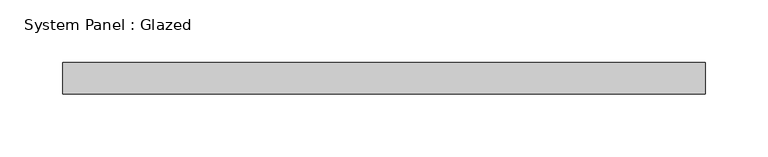
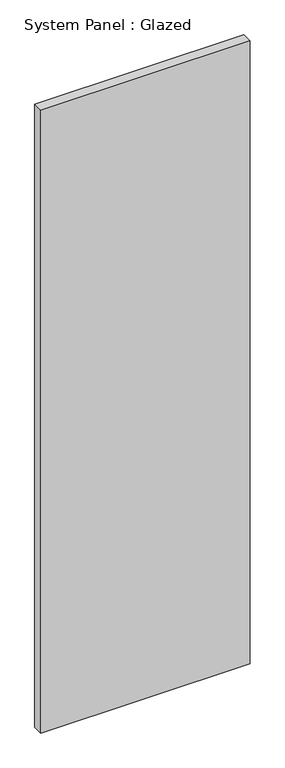
"""IFC4 building model written with IfcOpenShell, lengths in millimetres: plate geometry, System Panel : Glazed."""

from ifc_helpers import new_model, si_unit, origin, origin_with_axes, place, context, project, spatial, polyline, outline, extrude, source, transform, mapped, element, save


def system_panel_glazed_52b4f5c1(model_context):
    return source(origin(), model_context, "Body", "SweptSolid", [
        extrude(outline(polyline([(257.175, 19.05), (-257.175, 19.05), (-257.175, 44.45), (257.175, 44.45), (257.175, 19.05)])), origin_with_axes(), (0.0, 0.0, 1.0), 1617.0799136),
    ])


if __name__ == "__main__":
    model = new_model("IFC4")
    model_context = context("Model", 3, world=origin())
    ifc_project = project(units=[si_unit("LENGTHUNIT", "METRE", prefix="MILLI")], contexts=[model_context])
    site = spatial("IfcSite", under=ifc_project)
    building = spatial("IfcBuilding", under=site)
    placement = place(None, origin())
    system_panel_glazed_shape = system_panel_glazed_52b4f5c1(model_context)
    element("IfcPlate", 1, ObjectType="System Panel : Glazed", at=placement, inside=building, context=model_context, shape_type="MappedRepresentation", body=[
        mapped(system_panel_glazed_shape, transform((0.0, 0.0, 0.0), x_axis=(1.0, 0.0, 0.0), y_axis=(0.0, 1.0, 0.0), z_axis=(0.0, 0.0, 1.0))),
    ])
    save(model, "model.ifc")

# Revit data of these elements
# Type "System Panel : Glazed"
#   Construction Type Id = "GSP4R"
#   Analytic Construction = "1/8 in Pilkington single glazing"
#   Visual Light Transmittance = 0.9
#   Solar Heat Gain Coefficient = 0.86
#   Heat Transfer Coefficient (U) = 1.18115 BTU/(h·ft²·°F)
#   Define Thermal Properties by = 1
# Element 1 (IfcPlate, "System Panel : Glazed")
#   Materials on its faces: "Glass"
# Materials
#   "Glass": class "Glass", colour RGB 0 128 192, transparency 0.75, Description = "Soda Lime Glass", Cost = 0
